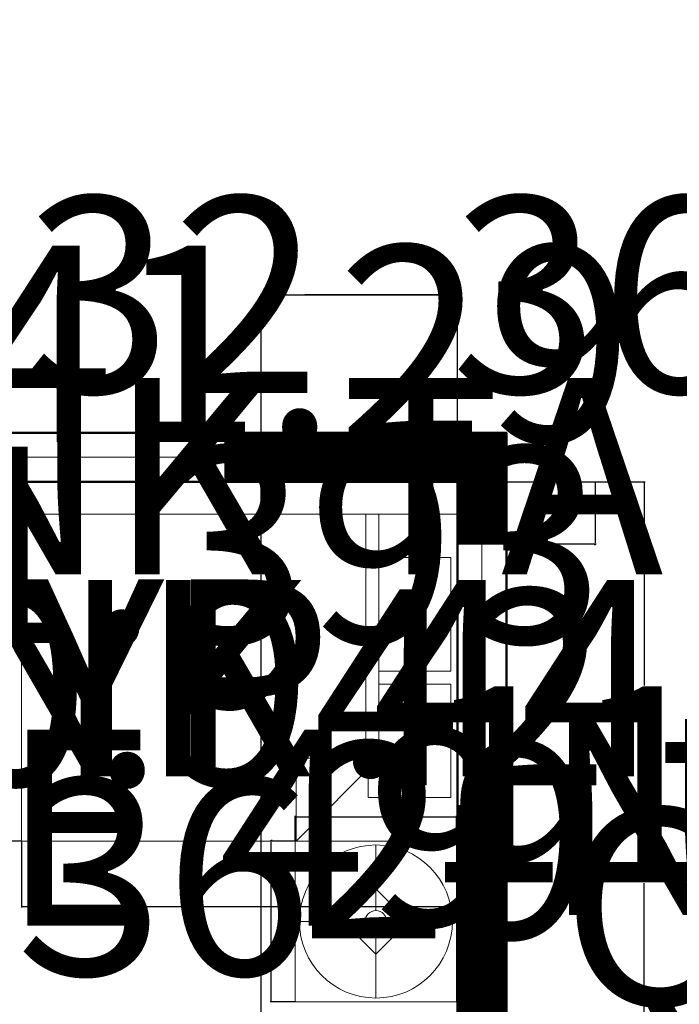
# Model space of a CAD drawing. Units: inches. Extents: x 1173 to 2157, y 515 to 1129.
# Tile 11 of 13: x 1581 to 1702, y 948 to 1129. Entities that reach past the tile are written whole.
import ezdxf

# ---------------------------------------------------------------- set-up
doc = ezdxf.new("R2010")
doc.units = ezdxf.units.IN
doc.header["$MEASUREMENT"] = 0
for name, color, linetype, lineweight in [('A-ANNO-DIMS', 2, 'Continuous', 18), ('A-FURN', 8, 'Continuous', 18), ('A-GLAZ', 4, 'Continuous', 18), ('A-WALL', 7, 'Continuous', 50)]:
    doc.layers.add(name, color=color, linetype=linetype, lineweight=lineweight)
doc.layers.add('A-WALL-PATT', color=22, linetype='Continuous', lineweight=13, true_color=0xca4b0c)
doc.styles.get("Standard").update_dxf_attribs({"font": 'arial.ttf'})
doc.dimstyles.get("Standard").update_dxf_attribs({"dimtxt": 36, "dimasz": 0.18, "dimexe": 0.18, "dimexo": 0.0625, "dimgap": 0.09, "dimtad": 0, "dimtih": 1, "dimtoh": 1, "dimdec": 0, "dimrnd": 72, "dimzin": 0, "dimdsep": 46, "dimlunit": 3, "dimtxsty": 'Standard', "dimcen": 2, "dimadec": 0, "dimazin": 0, "dimtfac": 1, "dimtdec": 0, "dimtofl": 0, "dimtmove": 0, "dimatfit": 3, "dimfxl": 1, "dimtolj": 1, "dimtzin": 0, "dimarcsym": 0})

# ---------------------------------------------------------------- blocks, each defined once
blk = doc.blocks.new('Bed - Queen')
for p, q in [((0, -80.00003), (0, 0)), ((0, 0), (59.99999, 0)), ((59.99999, 0), (59.99999, -80.00003)), ((7.99999, -1.2), (28.79998, -1.2)), ((7.99999, -14.4), (7.99999, -1.2)), ((28.79998, -1.2), (28.79998, -14.4)), ((31.19999, -1.2), (51.99999, -1.2)), ((31.19999, -14.4), (31.19999, -1.2)), ((51.99999, -1.2), (51.99999, -16.4)), ((0, -14.4), (44.8, -14.4)), ((59.99999, -29.6), (44.8, -14.4)), ((44.8, -14.4), (44.8, -29.6)), ((44.8, -16.8), (0, -16.8)), ((51.99999, -16.4), (46.79936, -16.4)), ((44.8, -29.6), (59.99999, -29.6)), ((59.99999, -80.00003), (0, -80.00003))]:
    blk.add_line(p, q)
blk = doc.blocks.new('Lamp - Table')
for p, q in [((0, 7), (0, 1)), ((0, 3), (-3, 0)), ((3, 0), (0, 3)), ((-1, 0), (-7, 0)), ((-3, 0), (0, -3)), ((0, -3), (3, 0)), ((1, 0), (7, 0)), ((0, -1), (0, -7))]:
    blk.add_line(p, q)
for radius in [7, 1]:
    blk.add_circle((0, 0), radius)
blk = doc.blocks.new('WIN-48X9')
blk.add_line((48, 4.5), (0, 4.5))
blk.add_lwpolyline([(0, 9), (48, 9), (48, 0), (0, 0)], close=True)
blk = doc.blocks.new('BEDROOM-NIGHTSTAND')
blk.add_lwpolyline([(29.6, 29.48), (0, 29.48), (0, 0), (29.6, 0)], close=True)
blk = doc.blocks.new('*D28')
at = {"layer": 'A-ANNO-DIMS', "color": 0, "lineweight": -2, "transparency": 16777216}
for p, q in [((1581.66, 978.31), (1581.66, 966.19)), ((1661.66, 978.31), (1661.66, 966.19)), ((1581.84, 966.37), (1661.48, 966.37)), ((1661.66, 966.37), (1661.84, 966.37))]:
    blk.add_line(p, q, dxfattribs=at)
at = {"layer": 'A-ANNO-DIMS', "color": 0, "transparency": 16777216}
for points in [[(1581.84, 966.4), (1581.84, 966.34), (1581.66, 966.37)], [(1661.48, 966.4), (1661.48, 966.34), (1661.66, 966.37)]]:
    blk.add_solid(points, dxfattribs=at)
at = {"layer": 'Defpoints', "color": 0, "transparency": 16777216}
for p in [(1581.66, 978.37), (1661.66, 978.37), (1661.66, 966.37)]:
    blk.add_point(p, dxfattribs=at)
at = {"layer": 'A-ANNO-DIMS', "color": 0, "transparency": 16777216, "insert": (1904.61, 966.37), "char_height": 36, "attachment_point": 5}
blk.add_mtext('\\A1;QUEEN BED 80 TYP.', dxfattribs=at)
blk = doc.blocks.new('*D29')
at = {"layer": 'A-ANNO-DIMS', "color": 0, "lineweight": -2, "transparency": 16777216}
for p, q in [((1581.6, 1038.37), (1569.48, 1038.37)), ((1569.66, 1038.19), (1569.66, 1026.84)), ((1569.66, 978.55), (1569.66, 989.9)), ((1581.6, 978.37), (1569.48, 978.37))]:
    blk.add_line(p, q, dxfattribs=at)
at = {"layer": 'A-ANNO-DIMS', "color": 0, "transparency": 16777216}
for points in [[(1569.63, 1038.19), (1569.69, 1038.19), (1569.66, 1038.37)], [(1569.63, 978.55), (1569.69, 978.55), (1569.66, 978.37)]]:
    blk.add_solid(points, dxfattribs=at)
at = {"layer": 'Defpoints', "color": 0, "transparency": 16777216}
for p in [(1581.66, 1038.37), (1569.66, 978.37), (1581.66, 978.37)]:
    blk.add_point(p, dxfattribs=at)
at = {"layer": 'A-ANNO-DIMS', "color": 0, "transparency": 16777216, "insert": (1569.66, 1008.37), "char_height": 36, "attachment_point": 5}
blk.add_mtext('\\A1;60 TYP.', dxfattribs=at)
blk = doc.blocks.new('*D34')
at = {"layer": 'A-ANNO-DIMS', "color": 0, "lineweight": -2, "transparency": 16777216}
for p, q in [((1631.9, 978.41), (1631.9, 982.97)), ((1661.5, 978.41), (1661.5, 982.97)), ((1632.08, 982.79), (1661.32, 982.79)), ((1661.5, 982.79), (1661.68, 982.79))]:
    blk.add_line(p, q, dxfattribs=at)
at = {"layer": 'A-ANNO-DIMS', "color": 0, "transparency": 16777216}
for points in [[(1632.08, 982.82), (1632.08, 982.76), (1631.9, 982.79)], [(1661.32, 982.82), (1661.32, 982.76), (1661.5, 982.79)]]:
    blk.add_solid(points, dxfattribs=at)
at = {"layer": 'Defpoints', "color": 0, "transparency": 16777216}
for p in [(1661.5, 982.79), (1631.9, 978.35), (1661.5, 978.35)]:
    blk.add_point(p, dxfattribs=at)
at = {"layer": 'A-ANNO-DIMS', "color": 0, "transparency": 16777216, "insert": (1918.96, 982.79), "char_height": 36, "attachment_point": 5}
blk.add_mtext('\\A1;NIGHTSTAND 30 TYP.', dxfattribs=at)
blk = doc.blocks.new('*D35')
at = {"layer": 'A-ANNO-DIMS', "color": 0, "lineweight": -2, "transparency": 16777216}
for p, q in [((1631.84, 978.35), (1627.28, 978.35)), ((1627.46, 978.35), (1627.46, 978.53)), ((1627.46, 978.53), (1627.64, 978.53)), ((1627.46, 949.05), (1627.46, 978.17)), ((1631.84, 948.87), (1627.28, 948.87))]:
    blk.add_line(p, q, dxfattribs=at)
at = {"layer": 'A-ANNO-DIMS', "color": 0, "transparency": 16777216}
for points in [[(1627.43, 978.17), (1627.49, 978.17), (1627.46, 978.35)], [(1627.43, 949.05), (1627.49, 949.05), (1627.46, 948.87)]]:
    blk.add_solid(points, dxfattribs=at)
at = {"layer": 'Defpoints', "color": 0, "transparency": 16777216}
for p in [(1627.46, 978.35), (1631.9, 978.35), (1631.9, 948.87)]:
    blk.add_point(p, dxfattribs=at)
at = {"layer": 'A-ANNO-DIMS', "color": 0, "transparency": 16777216, "insert": (1715.66, 978.53), "char_height": 36, "attachment_point": 5}
blk.add_mtext('\\A1;29 TYP.', dxfattribs=at)
blk = doc.blocks.new('*D36')
at = {"layer": 'A-ANNO-DIMS', "color": 0, "lineweight": -2, "transparency": 16777216}
for p, q in [((1497.87, 905.02), (1487.37, 905.02)), ((1487.55, 904.84), (1487.55, 889.09)), ((1487.55, 835.93), (1487.55, 851.68)), ((1497.87, 835.75), (1487.37, 835.75))]:
    blk.add_line(p, q, dxfattribs=at)
at = {"layer": 'A-ANNO-DIMS', "color": 0, "transparency": 16777216}
for points in [[(1487.52, 904.84), (1487.58, 904.84), (1487.55, 905.02)], [(1487.52, 835.93), (1487.58, 835.93), (1487.55, 835.75)]]:
    blk.add_solid(points, dxfattribs=at)
at = {"layer": 'Defpoints', "color": 0, "transparency": 16777216}
for p in [(1497.94, 905.02), (1487.55, 835.75), (1497.94, 835.75)]:
    blk.add_point(p, dxfattribs=at)
at = {"layer": 'A-ANNO-DIMS', "color": 0, "transparency": 16777216, "insert": (1487.55, 870.38), "char_height": 36, "attachment_point": 5}
blk.add_mtext('\\A1;DINING SET 69', dxfattribs=at)
blk = doc.blocks.new('*D46')
at = {"layer": 'A-ANNO-DIMS', "color": 0, "lineweight": -2, "transparency": 16777216}
for p, q in [((1646.37, 911.98), (1645.86, 896.32)), ((1648.72, 912.09), (1646.2, 912.17)), ((1648.2, 896.07), (1645.68, 896.15)), ((1645.86, 896.14), (1645.85, 895.96)), ((1645.85, 895.96), (1645.67, 895.96))]:
    blk.add_line(p, q, dxfattribs=at)
at = {"layer": 'A-ANNO-DIMS', "color": 0, "transparency": 16777216}
for points in [[(1646.34, 911.99), (1646.4, 911.98), (1646.38, 912.16)], [(1645.83, 896.32), (1645.89, 896.32), (1645.86, 896.14)]]:
    blk.add_solid(points, dxfattribs=at)
at = {"layer": 'Defpoints', "color": 0, "transparency": 16777216}
for p in [(1648.78, 912.09), (1645.86, 896.14), (1648.26, 896.06)]:
    blk.add_point(p, dxfattribs=at)
at = {"layer": 'A-ANNO-DIMS', "color": 0, "transparency": 16777216, "insert": (1538.16, 895.96), "char_height": 36, "attachment_point": 5}
blk.add_mtext('\\A1;BASIN 16', dxfattribs=at)
blk = doc.blocks.new('*D54')
at = {"layer": 'A-ANNO-DIMS', "color": 0, "lineweight": -2, "transparency": 16777216}
for p, q in [((1496.35, 1005.18), (1488.93, 1005.18)), ((1489.11, 1005), (1489.11, 999.54)), ((1489.11, 956.65), (1489.11, 962.11)), ((1496.35, 956.47), (1488.93, 956.47))]:
    blk.add_line(p, q, dxfattribs=at)
at = {"layer": 'A-ANNO-DIMS', "color": 0, "transparency": 16777216}
for points in [[(1489.08, 1005), (1489.14, 1005), (1489.11, 1005.18)], [(1489.08, 956.65), (1489.14, 956.65), (1489.11, 956.47)]]:
    blk.add_solid(points, dxfattribs=at)
at = {"layer": 'Defpoints', "color": 0, "transparency": 16777216}
for p in [(1496.42, 1005.18), (1489.11, 956.47), (1496.42, 956.47)]:
    blk.add_point(p, dxfattribs=at)
at = {"layer": 'A-ANNO-DIMS', "color": 0, "transparency": 16777216, "insert": (1489.11, 980.83), "char_height": 36, "attachment_point": 5}
blk.add_mtext('\\A1;WORK TABLE 49', dxfattribs=at)
blk = doc.blocks.new('*D58')
at = {"layer": 'A-ANNO-DIMS', "color": 0, "lineweight": -2, "transparency": 16777216}
for p, q in [((1476.55, 1014.81), (1476.55, 1008.07)), ((1520.66, 1014.81), (1520.66, 1008.07)), ((1476.73, 1008.25), (1520.48, 1008.25)), ((1520.66, 1008.25), (1520.84, 1008.25))]:
    blk.add_line(p, q, dxfattribs=at)
at = {"layer": 'A-ANNO-DIMS', "color": 0, "transparency": 16777216}
for points in [[(1476.73, 1008.28), (1476.73, 1008.22), (1476.55, 1008.25)], [(1520.48, 1008.28), (1520.48, 1008.22), (1520.66, 1008.25)]]:
    blk.add_solid(points, dxfattribs=at)
at = {"layer": 'Defpoints', "color": 0, "transparency": 16777216}
for p in [(1476.55, 1014.87), (1520.66, 1014.87), (1520.66, 1008.25)]:
    blk.add_point(p, dxfattribs=at)
at = {"layer": 'A-ANNO-DIMS', "color": 0, "transparency": 16777216, "insert": (1612.23, 1008.25), "char_height": 36, "attachment_point": 5}
blk.add_mtext('\\A1;SINK 44', dxfattribs=at)
blk = doc.blocks.new('*D60')
at = {"layer": 'A-ANNO-DIMS', "color": 0, "lineweight": -2, "transparency": 16777216}
for p, q in [((1396.06, 971.62), (1390.55, 971.62)), ((1390.73, 971.62), (1390.73, 971.8)), ((1390.73, 971.8), (1390.91, 971.8)), ((1390.73, 935.8), (1390.73, 971.44)), ((1396.06, 935.62), (1390.55, 935.62))]:
    blk.add_line(p, q, dxfattribs=at)
at = {"layer": 'A-ANNO-DIMS', "color": 0, "transparency": 16777216}
for points in [[(1390.7, 971.44), (1390.76, 971.44), (1390.73, 971.62)], [(1390.7, 935.8), (1390.76, 935.8), (1390.73, 935.62)]]:
    blk.add_solid(points, dxfattribs=at)
at = {"layer": 'Defpoints', "color": 0, "transparency": 16777216}
for p in [(1390.73, 971.62), (1396.13, 971.62), (1396.13, 935.62)]:
    blk.add_point(p, dxfattribs=at)
at = {"layer": 'A-ANNO-DIMS', "color": 0, "transparency": 16777216, "insert": (1517.73, 971.8), "char_height": 36, "attachment_point": 5}
blk.add_mtext('\\A1;FRIDGE 36', dxfattribs=at)
blk = doc.blocks.new('*D62')
at = {"layer": 'A-ANNO-DIMS', "color": 0, "lineweight": -2, "transparency": 16777216}
for p, q in [((1491.7, 1042.71), (1491.7, 1045.52)), ((1491.88, 1045.34), (1509.47, 1045.34)), ((1509.65, 1042.71), (1509.65, 1045.52)), ((1509.65, 1045.34), (1509.83, 1045.34))]:
    blk.add_line(p, q, dxfattribs=at)
at = {"layer": 'A-ANNO-DIMS', "color": 0, "transparency": 16777216}
for points in [[(1491.88, 1045.37), (1491.88, 1045.31), (1491.7, 1045.34)], [(1509.47, 1045.37), (1509.47, 1045.31), (1509.65, 1045.34)]]:
    blk.add_solid(points, dxfattribs=at)
at = {"layer": 'Defpoints', "color": 0, "transparency": 16777216}
for p in [(1509.65, 1045.34), (1491.7, 1042.65), (1509.65, 1042.65)]:
    blk.add_point(p, dxfattribs=at)
at = {"layer": 'A-ANNO-DIMS', "color": 0, "transparency": 16777216, "insert": (1657.22, 1045.34), "char_height": 36, "attachment_point": 5}
blk.add_mtext('\\A1;SINK TAP 18', dxfattribs=at)
blk = doc.blocks.new('*D88')
at = {"layer": 'A-ANNO-DIMS', "color": 0, "lineweight": -2, "transparency": 16777216}
for p, q in [((1529.66, 1044.34), (1529.65, 1069.76)), ((1529.83, 1069.58), (1570.76, 1069.61)), ((1570.95, 1044.37), (1570.94, 1069.79)), ((1570.94, 1069.61), (1571.12, 1069.61))]:
    blk.add_line(p, q, dxfattribs=at)
at = {"layer": 'A-ANNO-DIMS', "color": 0, "transparency": 16777216}
for points in [[(1529.83, 1069.61), (1529.83, 1069.55), (1529.65, 1069.58)], [(1570.76, 1069.64), (1570.76, 1069.58), (1570.94, 1069.61)]]:
    blk.add_solid(points, dxfattribs=at)
at = {"layer": 'Defpoints', "color": 0, "transparency": 16777216}
for p in [(1570.94, 1069.61), (1529.66, 1044.28), (1570.95, 1044.31)]:
    blk.add_point(p, dxfattribs=at)
at = {"layer": 'A-ANNO-DIMS', "color": 0, "transparency": 16777216, "insert": (1632.71, 1069.61), "char_height": 36, "attachment_point": 5}
blk.add_mtext('\\A1;41.29', dxfattribs=at)
blk = doc.blocks.new('*D89')
at = {"layer": 'A-ANNO-DIMS', "color": 0, "lineweight": -2, "transparency": 16777216}
for p, q in [((1529.66, 1044.34), (1529.66, 1078.79)), ((1529.84, 1078.61), (1557.68, 1078.61)), ((1661.48, 1078.61), (1633.64, 1078.61)), ((1661.66, 1044.34), (1661.66, 1078.79))]:
    blk.add_line(p, q, dxfattribs=at)
at = {"layer": 'A-ANNO-DIMS', "color": 0, "transparency": 16777216}
for points in [[(1529.84, 1078.64), (1529.84, 1078.58), (1529.66, 1078.61)], [(1661.48, 1078.64), (1661.48, 1078.58), (1661.66, 1078.61)]]:
    blk.add_solid(points, dxfattribs=at)
at = {"layer": 'Defpoints', "color": 0, "transparency": 16777216}
for p in [(1661.66, 1078.61), (1529.66, 1044.28), (1661.66, 1044.28)]:
    blk.add_point(p, dxfattribs=at)
at = {"layer": 'A-ANNO-DIMS', "color": 0, "transparency": 16777216, "insert": (1595.66, 1078.61), "char_height": 36, "attachment_point": 5}
blk.add_mtext('\\A1;132', dxfattribs=at)
blk = doc.blocks.new('*D90')
at = {"layer": 'A-ANNO-DIMS', "color": 0, "lineweight": -2, "transparency": 16777216}
for p, q in [((1661.73, 1044.28), (1696.15, 1044.28)), ((1695.97, 1044.1), (1695.97, 1006.94)), ((1695.97, 933.46), (1695.97, 970.62)), ((1625.73, 933.28), (1696.15, 933.28))]:
    blk.add_line(p, q, dxfattribs=at)
at = {"layer": 'A-ANNO-DIMS', "color": 0, "transparency": 16777216}
for points in [[(1695.94, 1044.1), (1696, 1044.1), (1695.97, 1044.28)], [(1695.94, 933.46), (1696, 933.46), (1695.97, 933.28)]]:
    blk.add_solid(points, dxfattribs=at)
at = {"layer": 'Defpoints', "color": 0, "transparency": 16777216}
for p in [(1661.66, 1044.28), (1625.66, 933.28), (1695.97, 933.28)]:
    blk.add_point(p, dxfattribs=at)
at = {"layer": 'A-ANNO-DIMS', "color": 0, "transparency": 16777216, "insert": (1695.97, 988.78), "char_height": 36, "attachment_point": 5}
blk.add_mtext('\\A1;111', dxfattribs=at)
blk = doc.blocks.new('*D91')
at = {"layer": 'A-ANNO-DIMS', "color": 0, "lineweight": -2, "transparency": 16777216}
for p, q in [((1661.73, 1044.28), (1687.15, 1044.28)), ((1686.97, 1044.1), (1686.97, 1033.07)), ((1661.73, 1032.89), (1687.15, 1032.89)), ((1686.97, 1032.71), (1686.79, 1032.71)), ((1686.97, 1032.89), (1686.97, 1032.71))]:
    blk.add_line(p, q, dxfattribs=at)
at = {"layer": 'A-ANNO-DIMS', "color": 0, "transparency": 16777216}
for points in [[(1686.94, 1044.1), (1687, 1044.1), (1686.97, 1044.28)], [(1686.94, 1033.07), (1687, 1033.07), (1686.97, 1032.89)]]:
    blk.add_solid(points, dxfattribs=at)
at = {"layer": 'Defpoints', "color": 0, "transparency": 16777216}
for p in [(1661.66, 1044.28), (1661.66, 1032.89), (1686.97, 1032.89)]:
    blk.add_point(p, dxfattribs=at)
at = {"layer": 'A-ANNO-DIMS', "color": 0, "transparency": 16777216, "insert": (1613.66, 1032.71), "char_height": 36, "attachment_point": 5}
blk.add_mtext('\\A1;11.393', dxfattribs=at)
blk = doc.blocks.new('*D98')
at = {"layer": 'A-ANNO-DIMS', "color": 0, "lineweight": -2, "transparency": 16777216}
for p, q in [((1625.66, 924.34), (1625.66, 1078.79)), ((1625.84, 1078.61), (1661.48, 1078.61)), ((1661.66, 924.34), (1661.66, 1078.79)), ((1661.66, 1078.61), (1661.84, 1078.61))]:
    blk.add_line(p, q, dxfattribs=at)
at = {"layer": 'A-ANNO-DIMS', "color": 0, "transparency": 16777216}
for points in [[(1625.84, 1078.64), (1625.84, 1078.58), (1625.66, 1078.61)], [(1661.48, 1078.64), (1661.48, 1078.58), (1661.66, 1078.61)]]:
    blk.add_solid(points, dxfattribs=at)
at = {"layer": 'Defpoints', "color": 0, "transparency": 16777216}
for p in [(1661.66, 1078.61), (1625.66, 924.28), (1661.66, 924.28)]:
    blk.add_point(p, dxfattribs=at)
at = {"layer": 'A-ANNO-DIMS', "color": 0, "transparency": 16777216, "insert": (1687.69, 1078.61), "char_height": 36, "attachment_point": 5}
blk.add_mtext('\\A1;36', dxfattribs=at)
blk = doc.blocks.new('*D107')
at = {"layer": 'A-ANNO-DIMS', "color": 0, "lineweight": -2, "transparency": 16777216}
for p, q in [((1607.48, 928.68), (1607.66, 928.68)), ((1607.66, 928.68), (1607.66, 920.46)), ((1607.66, 904.28), (1607.66, 908.28)), ((1605.66, 906.28), (1609.66, 906.28))]:
    blk.add_line(p, q, dxfattribs=at)
at = {"layer": 'A-ANNO-DIMS', "color": 0, "transparency": 16777216}
blk.add_solid([(1607.69, 920.46), (1607.63, 920.46), (1607.66, 920.28)], dxfattribs=at)
at = {"layer": 'Defpoints', "color": 0, "transparency": 16777216}
for p in [(1607.66, 920.28), (1607.66, 906.28)]:
    blk.add_point(p, dxfattribs=at)
at = {"layer": 'A-ANNO-DIMS', "color": 0, "transparency": 16777216, "insert": (1564.46, 928.68), "char_height": 36, "attachment_point": 5}
blk.add_mtext('\\A1;R14', dxfattribs=at)
blk = doc.blocks.new('*D110')
at = {"layer": 'A-ANNO-DIMS', "color": 0, "lineweight": -2, "transparency": 16777216}
for p, q in [((1415.92, 1004.58), (1415.92, 1008.58)), ((1413.92, 1006.58), (1417.92, 1006.58)), ((1424.67, 1006.58), (1421.57, 1006.58))]:
    blk.add_line(p, q, dxfattribs=at)
at = {"layer": 'A-ANNO-DIMS', "color": 0, "transparency": 16777216}
blk.add_solid([(1421.57, 1006.61), (1421.57, 1006.55), (1421.39, 1006.58)], dxfattribs=at)
at = {"layer": 'Defpoints', "color": 0, "transparency": 16777216}
for p in [(1410.45, 1006.58), (1421.39, 1006.58)]:
    blk.add_point(p, dxfattribs=at)
at = {"layer": 'A-ANNO-DIMS', "color": 0, "transparency": 16777216, "insert": (1556.91, 1006.58), "char_height": 36, "attachment_point": 5}
blk.add_mtext('\\A1;2X ∅10.942', dxfattribs=at)

msp = doc.modelspace()

# ---------------------------------------------------------------- hatches: boundary and pattern name
at = {"layer": 'A-WALL-PATT'}
h = msp.add_hatch(dxfattribs=at)
h.set_pattern_fill('ANSI31', color=256)
h.paths.add_polyline_path([(1388.6635, 933.2805), (1388.6635, 1044.2805), (1413.7618, 1044.2805), (1413.7618, 1053.2805), (1379.6635, 1053.2805), (1379.6635, 894.1606), (1388.6635, 894.1606), (1388.6635, 924.2805), (1472.6635, 924.2805), (1472.6635, 933.2805)])
h.paths.add_polyline_path([(1520.6635, 1044.2805), (1520.6635, 1014.7866), (1520.6635, 1005.1794), (1520.7714, 1005.1794), (1520.7714, 956.4707), (1520.6635, 924.2805), (1529.6635, 924.2805), (1529.6635, 931.4788), (1529.6635, 1044.2805), (1530.8474, 1044.2805), (1570.9543, 1044.2805), (1570.9543, 1053.2805), (1461.7618, 1053.2805), (1461.7618, 1044.2805)])
h.paths.add_polyline_path([(1618.9543, 1053.2805), (1618.9543, 1044.2805), (1661.6635, 1044.2805), (1661.6635, 1043.7367), (1661.6635, 1032.8874), (1670.6635, 1032.8874), (1670.6635, 1053.2805)])
h.paths.add_polyline_path([(1661.6635, 933.2805), (1661.6635, 927.8377), (1661.6635, 924.2805), (1661.6635, 918.9156), (1670.6635, 918.9156), (1670.6635, 984.8874), (1661.6635, 984.8874), (1661.6635, 978.3712)])
h.paths.add_polyline_path([(1670.6635, 894.9156), (1661.6635, 894.9156), (1661.6635, 890.0349), (1661.9328, 890.0349), (1661.9328, 870.079), (1661.6635, 864.2805), (1589.6635, 864.2805), (1589.6635, 924.2805), (1625.553, 924.2805, -0.02455299), (1625.3782, 927.8377), (1625.3782, 933.2805), (1577.6635, 933.2805), (1577.6635, 924.2805), (1580.6635, 924.2805), (1580.6635, 855.2805), (1586.1062, 855.2805), (1589.6635, 855.2805), (1661.6635, 855.2805), (1661.6635, 826.5597), (1670.6635, 826.5597)])
h.paths.add_polyline_path([(1670.6635, 802.5597), (1661.6635, 802.5597), (1661.6635, 795.2805), (1589.6635, 795.2805), (1589.6635, 819.17, -0.02455299), (1586.1062, 818.9952), (1580.6635, 818.9952), (1580.6635, 795.2805), (1577.6635, 795.2805), (1577.6635, 786.2805), (1661.6635, 786.2805), (1661.6635, 778.5597), (1661.6635, 742.6973), (1670.6635, 742.6973)])
h.paths.add_polyline_path([(1661.6635, 654.2805), (1625.1498, 654.2805), (1625.1498, 645.2805), (1661.3656, 645.2805), (1661.6635, 645.2805), (1661.6635, 573.2805), (1520.6635, 573.2805), (1520.6635, 564.2805), (1670.6635, 564.2805), (1670.6635, 694.6973), (1661.6635, 694.6973)])
h.paths.add_polyline_path([(1529.4367, 733.4702, -0.06854064), (1529.6635, 734.2623), (1529.6635, 795.2805), (1520.6635, 795.2805), (1520.6635, 645.2805), (1577.1498, 645.2805), (1577.1498, 654.2805), (1529.6635, 654.2805), (1529.6635, 686.5626, -0.06854064), (1529.4367, 687.3547)])
h.paths.add_polyline_path([(1379.6635, 711.2805), (1388.6635, 711.2805), (1458.7214, 711.2805), (1458.7214, 720.2805), (1410.7214, 720.2805), (1388.6635, 720.2805), (1388.6635, 745.0427), (1379.6635, 745.0427)])
h.paths.add_polyline_path([(1388.6635, 846.1606), (1379.6635, 846.1606), (1379.6635, 793.0427), (1388.6635, 793.0427)])

# ---------------------------------------------------------------- linework, layer by layer
at = {"layer": 'A-WALL'}
for p, q in [((1661.6635, 1044.2805), (1529.6635, 1044.2805)), ((1661.6635, 933.2805), (1661.6635, 1044.2805)), ((1661.6635, 1043.7367), (1661.6635, 1044.2805))]:
    msp.add_line(p, q, dxfattribs=at)
msp.add_lwpolyline([(1379.6635, 564.2805), (1670.6635, 564.2805), (1670.6635, 1053.2805), (1379.6635, 1053.2805)], close=True, dxfattribs=at)

# ---------------------------------------------------------------- block references
at = {"layer": 'A-FURN', "rotation": 270}
msp.add_blockref('Bed - Queen', (1661.6635, 1038.3712), dxfattribs=at)
at = {"layer": 'A-FURN'}
msp.add_blockref('BEDROOM-NIGHTSTAND', (1631.9047, 948.8672), dxfattribs=at)
at = {"layer": 'A-FURN', "xscale": 2.006708061362473, "yscale": 2.006708061362473, "zscale": 2.006708061362473}
msp.add_blockref('Lamp - Table', (1646.7047, 963.6096), dxfattribs=at)
at = {"layer": 'A-GLAZ'}
msp.add_blockref('WIN-48X9', (1570.9543, 1044.3102), dxfattribs=at)
at = {"layer": 'A-GLAZ', "rotation": 270.0000000000009}
msp.add_blockref('WIN-48X9', (1661.6635, 1032.8874), dxfattribs=at)

# ---------------------------------------------------------------- dimensions: what is measured, and where the dimension line sits
at = {"layer": 'A-ANNO-DIMS'}
for base, p1, p2, text, picture, middle in [((1509.6463, 1045.3406), (1491.6951, 1042.6479), (1509.6463, 1042.6479), 'SINK TAP <>', '*D62', (1657.2192, 1045.3406)), ((1661.6635, 966.3712), (1581.6634, 978.3712), (1661.6635, 978.3712), 'QUEEN BED <> TYP.', '*D28', (1904.6142, 966.3712)), ((1661.5047, 982.7919), (1631.9047, 978.3519), (1661.5047, 978.3519), 'NIGHTSTAND <> TYP.', '*D34', (1918.9562, 982.7919)), ((1520.6635, 1008.2517), (1476.5465, 1014.8692), (1520.6635, 1014.8692), 'SINK <>', '*D58', (1612.235, 1008.2517))]:
    dim = msp.add_linear_dim(base=base, p1=p1, p2=p2, text=text, dimstyle='Standard', override={"dimdec": 0, "dimlfac": 1, "dimrnd": 0, "dimzin": 0, "dimdsep": 46, "dimlunit": 2}, dxfattribs=at)
    dim.commit()
    dim.dimension.update_dxf_attribs({"geometry": picture, "text_midpoint": middle})
for p1, p2, picture, middle in [((1529.6635, 1044.2805), (1661.6635, 1044.2805), '*D89', (1595.6635, 1078.6127)), ((1625.6635, 924.2805), (1661.6635, 924.2805), '*D98', (1687.6933, 1078.6127))]:
    dim = msp.add_linear_dim(base=(1661.6635, 1078.6127), p1=p1, p2=p2, dimstyle='Standard', override={"dimdec": 0, "dimlfac": 1, "dimrnd": 0, "dimzin": 0, "dimdsep": 46, "dimlunit": 2}, dxfattribs=at)
    dim.commit()
    dim.dimension.update_dxf_attribs({"geometry": picture, "text_midpoint": middle})
for base, p1, p2, angle, override, picture, middle in [((1570.9361, 1069.6126), (1529.6635, 1044.2805), (1570.9543, 1044.3102), 0.041121, {"dimdec": 2, "dimlfac": 1, "dimrnd": 0, "dimzin": 0, "dimdsep": 46, "dimlunit": 2}, '*D88', (1632.7082, 1069.6128)), ((1686.966, 1032.8874), (1661.6635, 1044.2805), (1661.6635, 1032.8874), 270, {"dimdec": 3, "dimlfac": 1, "dimrnd": 0, "dimzin": 0, "dimdsep": 46, "dimlunit": 2}, '*D91', (1613.6646, 1032.7074)), ((1695.966, 933.2805), (1661.6635, 1044.2805), (1625.6635, 933.2805), 90, {"dimdec": 0, "dimlfac": 1, "dimrnd": 0, "dimzin": 0, "dimdsep": 46, "dimlunit": 2}, '*D90', (1695.966, 988.7805))]:
    dim = msp.add_linear_dim(base=base, p1=p1, p2=p2, angle=angle, dimstyle='Standard', override=override, dxfattribs=at)
    dim.commit()
    dim.dimension.update_dxf_attribs({"geometry": picture, "text_midpoint": middle})
for base, p1, p2, angle, text, picture, middle in [((1489.1107, 956.4707), (1496.4171, 1005.1794), (1496.4171, 956.4707), 270, 'WORK TABLE <>', '*D54', (1489.1107, 980.8251)), ((1569.6634, 978.3712), (1581.6634, 1038.3712), (1581.6634, 978.3712), 270, '<> TYP.', '*D29', (1569.6634, 1008.3712)), ((1627.4647, 978.3519), (1631.9047, 948.8672), (1631.9047, 978.3519), 90, '<> TYP.', '*D35', (1715.6597, 978.5319)), ((1390.7251, 971.618), (1396.1251, 935.618), (1396.1251, 971.618), 90, 'FRIDGE <>', '*D60', (1517.7318, 971.798)), ((1487.5464, 835.7486), (1497.9367, 905.017), (1497.9367, 835.7486), 270, 'DINING SET <>', '*D36', (1487.5464, 870.3828)), ((1645.8589, 896.1412), (1648.7786, 912.0868), (1648.2623, 896.0638), 268.15447, 'BASIN <>', '*D46', (1538.1601, 895.9613))]:
    dim = msp.add_linear_dim(base=base, p1=p1, p2=p2, angle=angle, text=text, dimstyle='Standard', override={"dimdec": 0, "dimlfac": 1, "dimrnd": 0, "dimzin": 0, "dimdsep": 46, "dimlunit": 2}, dxfattribs=at)
    dim.commit()
    dim.dimension.update_dxf_attribs({"geometry": picture, "text_midpoint": middle})
dim = msp.add_diameter_dim_2p(p1=(1410.4482, 1006.5809), p2=(1421.3897, 1006.58), text='2X <>', dimstyle='Standard', override={"dimdec": 3, "dimlfac": 1, "dimrnd": 0, "dimzin": 0, "dimdsep": 46, "dimlunit": 2}, dxfattribs=at)
dim.commit()
dim.dimension.update_dxf_attribs({"geometry": '*D110', "text_midpoint": (1424.6722, 1006.5797), "dimtype": 163})
dim = msp.add_radius_dim(center=(1607.6635, 906.2805), mpoint=(1607.663, 920.2805), dimstyle='Standard', override={"dimdec": 0, "dimlfac": 1, "dimrnd": 0, "dimzin": 0, "dimdsep": 46, "dimlunit": 2}, dxfattribs=at)
dim.commit()
dim.dimension.update_dxf_attribs({"geometry": '*D107', "text_midpoint": (1564.4555, 928.6805), "dimtype": 164})

doc.saveas('drawing.dxf')
